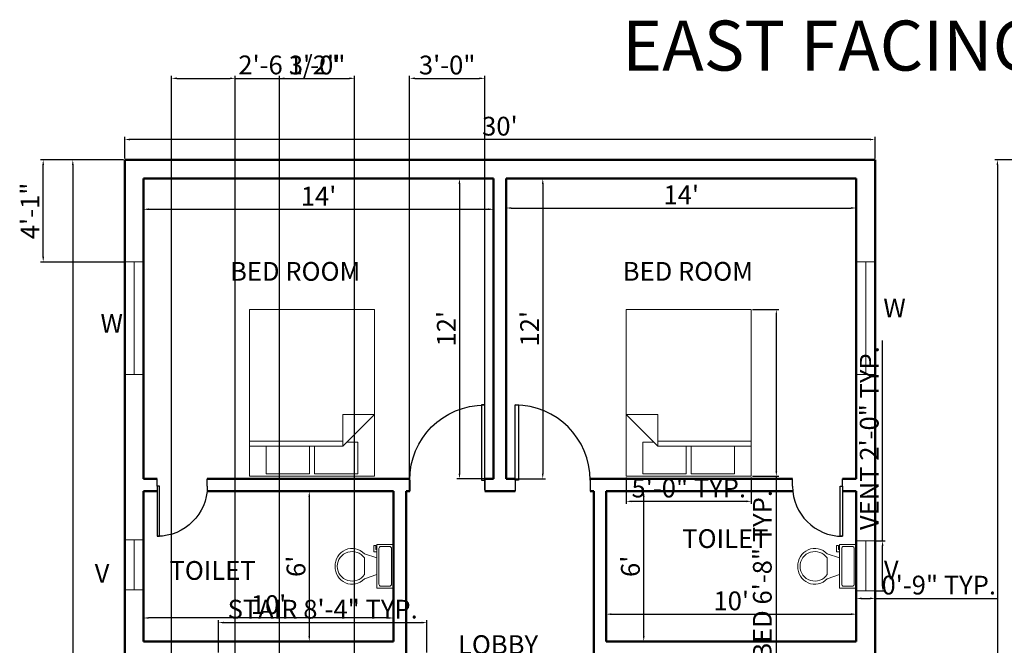
# Model space of a CAD drawing. Units: inches. Extents: x 3587 to 4539, y 1613 to 2440.
# Tile 6 of 8: x 3594 to 4067, y 2140 to 2440. Entities that reach past the tile are written whole.
import ezdxf

# ---------------------------------------------------------------- set-up
doc = ezdxf.new("R2010")
doc.units = ezdxf.units.IN
for name, color, linetype, lineweight in [('A-ANNO-DIMS', 2, 'Continuous', 18), ('A-ANNO-TEXT', 7, 'Continuous', 18), ('A-ANNO-TITL', 7, 'Continuous', 35), ('A-AREA-IDEN', 7, 'Continuous', 25), ('A-DOOR', 3, 'Continuous', 25), ('A-FLOR-FIXT', 9, 'Continuous', 18), ('A-FURN', 8, 'Continuous', 18), ('A-GLAZ', 4, 'Continuous', 20), ('A-WALL', 7, 'Continuous', 50)]:
    doc.layers.add(name, color=color, linetype=linetype, lineweight=lineweight)
doc.styles.get("Standard").update_dxf_attribs({"font": 'arial.ttf'})
doc.dimstyles.new('ISO-25', dxfattribs={"dimtxt": 9, "dimasz": 2.5, "dimexe": 1.25, "dimexo": 0.625, "dimtad": 1, "dimlunit": 3, "dimtxsty": 'Standard', "dimcen": 2.5, "dimadec": 0, "dimazin": 0, "dimtfac": 1, "dimtmove": 0, "dimatfit": 3, "dimfxl": 1, "dimarcsym": 0})

# ---------------------------------------------------------------- blocks, each defined once
blk = doc.blocks.new('*U4')
for p, q in [((0, 0), (0, -6)), ((40, 0), (40, -6))]:
    blk.add_line(p, q)
blk.add_lwpolyline([(0, 0), (0, 40), (1.75, 40), (1.75, 0)], close=True)
blk.add_arc((0, 0), 40, 0, 90)
blk = doc.blocks.new('*U11')
for p, q in [((9.5, -6), (9.5, -2)), ((-10, -8.5), (-8, -8.5)), ((-10, -9.5), (-10, -8.5)), ((-8, -8.5), (-8, -8)), ((-7, -8), (-7, -9.5)), ((-4, -8), (-6, -14)), ((4, -8), (6, -14)), ((-7, -9.5), (-10, -9.5)), ((4, -14), (-4, -14))]:
    blk.add_line(p, q)
blk.add_lwpolyline([(10.5, -8), (10.5, 0), (-10.5, 0), (-10.5, -8)], close=True)
for points in [[(-9.5, -2), (-9.5, -6)], [(8.5, -1), (-8.5, -1)], [(-8.5, -7), (8.5, -7)]]:
    blk.add_lwpolyline(points)
for centre, radius, start, end in [((-8.625, -1.875), 0.8839, 81.8699, 188.1301), ((8.625, -1.875), 0.8839, 351.8699, 98.1301), ((-8.625, -6.125), 0.8839, 171.869898, 278.1301), ((8.625, -6.125), 0.8839, 261.8699, 8.1301), ((-0.4772, -19.9188), 8.0953, 133.01722, 273.38), ((0.0374, -19.8731), 7.127, 124.50543, 269.7), ((-0.0373, -19.8731), 7.127, 270.3, 55.4946), ((0.4773, -19.9188), 8.0953, 266.62, 46.9828)]:
    blk.add_arc(centre, radius, start, end)
blk = doc.blocks.new('Bed - Queen')
for p, q in [((0, -80.00003), (0, 0)), ((0, 0), (59.99999, 0)), ((59.99999, 0), (59.99999, -80.00003)), ((7.99999, -1.2), (28.79998, -1.2)), ((7.99999, -14.4), (7.99999, -1.2)), ((28.79998, -1.2), (28.79998, -14.4)), ((31.19999, -1.2), (51.99999, -1.2)), ((31.19999, -14.4), (31.19999, -1.2)), ((51.99999, -1.2), (51.99999, -16.4)), ((0, -14.4), (44.8, -14.4)), ((44.8, -16.8), (0, -16.8)), ((59.99999, -29.6), (44.8, -14.4)), ((44.8, -14.4), (44.8, -29.6)), ((51.99999, -16.4), (46.79936, -16.4)), ((44.8, -29.6), (59.99999, -29.6)), ((59.99999, -80.00003), (0, -80.00003))]:
    blk.add_line(p, q)
blk = doc.blocks.new('*D13')
at = {"layer": 'A-ANNO-DIMS', "color": 0, "lineweight": -2, "transparency": 16777216}
for p, q in [((3644.52, 2373.56), (3644.52, 2383.96)), ((4002.02, 2382.71), (3647.02, 2382.71)), ((4004.52, 2373.56), (4004.52, 2383.96))]:
    blk.add_line(p, q, dxfattribs=at)
at = {"layer": 'A-ANNO-DIMS', "color": 0, "transparency": 16777216}
for points in [[(3647.02, 2383.12), (3647.02, 2382.29), (3644.52, 2382.71)], [(4002.02, 2383.12), (4002.02, 2382.29), (4004.52, 2382.71)]]:
    blk.add_solid(points, dxfattribs=at)
at = {"layer": 'Defpoints', "color": 0, "transparency": 16777216}
for p in [(3644.52, 2382.71), (3644.52, 2372.93), (4004.52, 2372.93)]:
    blk.add_point(p, dxfattribs=at)
at = {"layer": 'A-ANNO-DIMS', "color": 0, "transparency": 16777216, "insert": (3824.52, 2387.93), "char_height": 9, "attachment_point": 5}
blk.add_mtext("30'", dxfattribs=at)
blk = doc.blocks.new('*D14')
at = {"layer": 'A-ANNO-DIMS', "color": 0, "lineweight": -2, "transparency": 16777216}
for p, q in [((3643.9, 2372.93), (3618.39, 2372.93)), ((3619.64, 2370.43), (3619.64, 1655.43)), ((3643.9, 1652.93), (3618.39, 1652.93))]:
    blk.add_line(p, q, dxfattribs=at)
at = {"layer": 'A-ANNO-DIMS', "color": 0, "transparency": 16777216}
for points in [[(3619.22, 2370.43), (3620.05, 2370.43), (3619.64, 2372.93)], [(3619.22, 1655.43), (3620.05, 1655.43), (3619.64, 1652.93)]]:
    blk.add_solid(points, dxfattribs=at)
at = {"layer": 'Defpoints', "color": 0, "transparency": 16777216}
for p in [(3644.52, 2372.93), (3619.64, 1652.93), (3644.52, 1652.93)]:
    blk.add_point(p, dxfattribs=at)
at = {"layer": 'A-ANNO-DIMS', "color": 0, "transparency": 16777216, "insert": (3614.42, 2019.45), "char_height": 9, "attachment_point": 5, "rotation": 90}
blk.add_mtext("60'", dxfattribs=at)
blk = doc.blocks.new('*D15')
at = {"layer": 'A-ANNO-DIMS', "color": 0, "lineweight": -2, "transparency": 16777216}
for p, q in [((3653.52, 2363.31), (3653.52, 2347.98)), ((3821.52, 2363.31), (3821.52, 2347.98)), ((3656.02, 2349.23), (3819.02, 2349.23))]:
    blk.add_line(p, q, dxfattribs=at)
at = {"layer": 'A-ANNO-DIMS', "color": 0, "transparency": 16777216}
for points in [[(3656.02, 2349.64), (3656.02, 2348.81), (3653.52, 2349.23)], [(3819.02, 2349.64), (3819.02, 2348.81), (3821.52, 2349.23)]]:
    blk.add_solid(points, dxfattribs=at)
at = {"layer": 'Defpoints', "color": 0, "transparency": 16777216}
for p in [(3653.52, 2363.93), (3821.52, 2363.93), (3821.52, 2349.23)]:
    blk.add_point(p, dxfattribs=at)
at = {"layer": 'A-ANNO-DIMS', "color": 0, "transparency": 16777216, "insert": (3737.52, 2354.37), "char_height": 9, "attachment_point": 5}
blk.add_mtext("14'", dxfattribs=at)
blk = doc.blocks.new('*D16')
at = {"layer": 'A-ANNO-DIMS', "color": 0, "lineweight": -2, "transparency": 16777216}
for p, q in [((3820.9, 2363.93), (3803.88, 2363.93)), ((3805.13, 2361.43), (3805.13, 2222.43)), ((3820.9, 2219.93), (3803.88, 2219.93))]:
    blk.add_line(p, q, dxfattribs=at)
at = {"layer": 'A-ANNO-DIMS', "color": 0, "transparency": 16777216}
for points in [[(3804.72, 2361.43), (3805.55, 2361.43), (3805.13, 2363.93)], [(3804.72, 2222.43), (3805.55, 2222.43), (3805.13, 2219.93)]]:
    blk.add_solid(points, dxfattribs=at)
at = {"layer": 'Defpoints', "color": 0, "transparency": 16777216}
for p in [(3821.52, 2363.93), (3805.13, 2219.93), (3821.52, 2219.93)]:
    blk.add_point(p, dxfattribs=at)
at = {"layer": 'A-ANNO-DIMS', "color": 0, "transparency": 16777216, "insert": (3799.99, 2291.93), "char_height": 9, "attachment_point": 5, "rotation": 90}
blk.add_mtext("12'", dxfattribs=at)
blk = doc.blocks.new('*D17')
at = {"layer": 'A-ANNO-DIMS', "color": 0, "lineweight": -2, "transparency": 16777216}
for p, q in [((3827.52, 2363.31), (3827.52, 2348.58)), ((3995.52, 2363.31), (3995.52, 2348.58)), ((3830.02, 2349.83), (3993.02, 2349.83))]:
    blk.add_line(p, q, dxfattribs=at)
at = {"layer": 'A-ANNO-DIMS', "color": 0, "transparency": 16777216}
for points in [[(3830.02, 2350.25), (3830.02, 2349.41), (3827.52, 2349.83)], [(3993.02, 2350.25), (3993.02, 2349.41), (3995.52, 2349.83)]]:
    blk.add_solid(points, dxfattribs=at)
at = {"layer": 'Defpoints', "color": 0, "transparency": 16777216}
for p in [(3827.52, 2363.93), (3995.52, 2363.93), (3995.52, 2349.83)]:
    blk.add_point(p, dxfattribs=at)
at = {"layer": 'A-ANNO-DIMS', "color": 0, "transparency": 16777216, "insert": (3911.52, 2354.97), "char_height": 9, "attachment_point": 5}
blk.add_mtext("14'", dxfattribs=at)
blk = doc.blocks.new('*D18')
at = {"layer": 'A-ANNO-DIMS', "color": 0, "lineweight": -2, "transparency": 16777216}
for p, q in [((3828.15, 2363.93), (3846.35, 2363.93)), ((3845.1, 2361.43), (3845.1, 2222.43)), ((3828.15, 2219.93), (3846.35, 2219.93))]:
    blk.add_line(p, q, dxfattribs=at)
at = {"layer": 'A-ANNO-DIMS', "color": 0, "transparency": 16777216}
for points in [[(3844.68, 2361.43), (3845.51, 2361.43), (3845.1, 2363.93)], [(3844.68, 2222.43), (3845.51, 2222.43), (3845.1, 2219.93)]]:
    blk.add_solid(points, dxfattribs=at)
at = {"layer": 'Defpoints', "color": 0, "transparency": 16777216}
for p in [(3827.52, 2363.93), (3827.52, 2219.93), (3845.1, 2219.93)]:
    blk.add_point(p, dxfattribs=at)
at = {"layer": 'A-ANNO-DIMS', "color": 0, "transparency": 16777216, "insert": (3839.95, 2291.93), "char_height": 9, "attachment_point": 5, "rotation": 90}
blk.add_mtext("12'", dxfattribs=at)
blk = doc.blocks.new('*D19')
at = {"layer": 'A-ANNO-DIMS', "color": 0, "lineweight": -2, "transparency": 16777216}
for p, q in [((3653.52, 2142.56), (3653.52, 2154.41)), ((3773.52, 2142.56), (3773.52, 2154.41)), ((3771.02, 2153.16), (3656.02, 2153.16))]:
    blk.add_line(p, q, dxfattribs=at)
at = {"layer": 'A-ANNO-DIMS', "color": 0, "transparency": 16777216}
for points in [[(3656.02, 2153.58), (3656.02, 2152.75), (3653.52, 2153.16)], [(3771.02, 2153.58), (3771.02, 2152.75), (3773.52, 2153.16)]]:
    blk.add_solid(points, dxfattribs=at)
at = {"layer": 'Defpoints', "color": 0, "transparency": 16777216}
for p in [(3653.52, 2153.16), (3653.52, 2141.93), (3773.52, 2141.93)]:
    blk.add_point(p, dxfattribs=at)
at = {"layer": 'A-ANNO-DIMS', "color": 0, "transparency": 16777216, "insert": (3713.52, 2158.38), "char_height": 9, "attachment_point": 5}
blk.add_mtext("10'", dxfattribs=at)
blk = doc.blocks.new('*D20')
at = {"layer": 'A-ANNO-DIMS', "color": 0, "lineweight": -2, "transparency": 16777216}
for p, q in [((3772.9, 2213.93), (3731.83, 2213.93)), ((3733.08, 2211.43), (3733.08, 2144.43)), ((3772.9, 2141.93), (3731.83, 2141.93))]:
    blk.add_line(p, q, dxfattribs=at)
at = {"layer": 'A-ANNO-DIMS', "color": 0, "transparency": 16777216}
for points in [[(3732.67, 2211.43), (3733.5, 2211.43), (3733.08, 2213.93)], [(3732.67, 2144.43), (3733.5, 2144.43), (3733.08, 2141.93)]]:
    blk.add_solid(points, dxfattribs=at)
at = {"layer": 'Defpoints', "color": 0, "transparency": 16777216}
for p in [(3773.52, 2213.93), (3733.08, 2141.93), (3773.52, 2141.93)]:
    blk.add_point(p, dxfattribs=at)
at = {"layer": 'A-ANNO-DIMS', "color": 0, "transparency": 16777216, "insert": (3727.86, 2177.93), "char_height": 9, "attachment_point": 5, "rotation": 90}
blk.add_mtext("6'", dxfattribs=at)
blk = doc.blocks.new('*D21')
at = {"layer": 'A-ANNO-DIMS', "color": 0, "lineweight": -2, "transparency": 16777216}
for p, q in [((3876.15, 2213.93), (3894.78, 2213.93)), ((3893.53, 2144.43), (3893.53, 2211.43)), ((3876.15, 2141.93), (3894.78, 2141.93))]:
    blk.add_line(p, q, dxfattribs=at)
at = {"layer": 'A-ANNO-DIMS', "color": 0, "transparency": 16777216}
for points in [[(3893.12, 2211.43), (3893.95, 2211.43), (3893.53, 2213.93)], [(3893.12, 2144.43), (3893.95, 2144.43), (3893.53, 2141.93)]]:
    blk.add_solid(points, dxfattribs=at)
at = {"layer": 'Defpoints', "color": 0, "transparency": 16777216}
for p in [(3875.52, 2213.93), (3893.53, 2213.93), (3875.52, 2141.93)]:
    blk.add_point(p, dxfattribs=at)
at = {"layer": 'A-ANNO-DIMS', "color": 0, "transparency": 16777216, "insert": (3888.31, 2177.93), "char_height": 9, "attachment_point": 5, "rotation": 90}
blk.add_mtext("6'", dxfattribs=at)
blk = doc.blocks.new('*D22')
at = {"layer": 'A-ANNO-DIMS', "color": 0, "lineweight": -2, "transparency": 16777216}
for p, q in [((3875.52, 2142.56), (3875.52, 2156.23)), ((3878.02, 2154.98), (3993.02, 2154.98)), ((3995.52, 2142.56), (3995.52, 2156.23))]:
    blk.add_line(p, q, dxfattribs=at)
at = {"layer": 'A-ANNO-DIMS', "color": 0, "transparency": 16777216}
for points in [[(3878.02, 2155.4), (3878.02, 2154.56), (3875.52, 2154.98)], [(3993.02, 2155.4), (3993.02, 2154.56), (3995.52, 2154.98)]]:
    blk.add_solid(points, dxfattribs=at)
at = {"layer": 'Defpoints', "color": 0, "transparency": 16777216}
for p in [(3995.52, 2154.98), (3875.52, 2141.93), (3995.52, 2141.93)]:
    blk.add_point(p, dxfattribs=at)
at = {"layer": 'A-ANNO-DIMS', "color": 0, "transparency": 16777216, "insert": (3935.52, 2160.2), "char_height": 9, "attachment_point": 5}
blk.add_mtext("10'", dxfattribs=at)
blk = doc.blocks.new('*D28')
at = {"layer": 'A-ANNO-DIMS', "color": 0, "lineweight": -2, "transparency": 16777216}
for p, q in [((4087.49, 2372.93), (4061.98, 2372.93)), ((4063.23, 2370.43), (4063.23, 1655.43)), ((4087.49, 1652.93), (4061.98, 1652.93))]:
    blk.add_line(p, q, dxfattribs=at)
at = {"layer": 'A-ANNO-DIMS', "color": 0, "transparency": 16777216}
for points in [[(4062.81, 2370.43), (4063.65, 2370.43), (4063.23, 2372.93)], [(4062.81, 1655.43), (4063.65, 1655.43), (4063.23, 1652.93)]]:
    blk.add_solid(points, dxfattribs=at)
at = {"layer": 'Defpoints', "color": 0, "transparency": 16777216}
for p in [(4088.12, 2372.93), (4063.23, 1652.93), (4088.12, 1652.93)]:
    blk.add_point(p, dxfattribs=at)
at = {"layer": 'A-ANNO-DIMS', "color": 0, "transparency": 16777216, "insert": (4058.01, 2019.45), "char_height": 9, "attachment_point": 5, "rotation": 90}
blk.add_mtext("60'", dxfattribs=at)
blk = doc.blocks.new('WINDOW-54IN')
for p, q in [((9, 54), (0, 54)), ((4.5, 54), (4.5, 0)), ((9, 0), (0, 0))]:
    blk.add_line(p, q)
blk = doc.blocks.new('VENT-24IN')
for p, q in [((9, 24), (0, 24)), ((4.5, 0), (4.5, 24)), ((9, 0), (0, 0))]:
    blk.add_line(p, q)
blk = doc.blocks.new('*D56')
at = {"layer": 'A-ANNO-DIMS', "color": 0, "lineweight": -2, "transparency": 16777216}
for p, q in [((4008.12, 2190.14), (4008.12, 2286.24)), ((4005.15, 2190.14), (4009.37, 2190.14)), ((4008.12, 2168.64), (4008.12, 2187.64)), ((4005.15, 2166.14), (4009.37, 2166.14))]:
    blk.add_line(p, q, dxfattribs=at)
at = {"layer": 'A-ANNO-DIMS', "color": 0, "transparency": 16777216}
for points in [[(4007.71, 2187.64), (4008.54, 2187.64), (4008.12, 2190.14)], [(4007.71, 2168.64), (4008.54, 2168.64), (4008.12, 2166.14)]]:
    blk.add_solid(points, dxfattribs=at)
at = {"layer": 'Defpoints', "color": 0, "transparency": 16777216}
for p in [(4004.52, 2190.14), (4008.12, 2190.14), (4004.52, 2166.14)]:
    blk.add_point(p, dxfattribs=at)
at = {"layer": 'A-ANNO-DIMS', "color": 0, "transparency": 16777216, "insert": (4002.9, 2239.44), "char_height": 9, "attachment_point": 5, "rotation": 90}
blk.add_mtext('VENT 2\'-0" TYP.', dxfattribs=at)
blk = doc.blocks.new('*D57')
at = {"layer": 'A-ANNO-DIMS', "color": 0, "lineweight": -2, "transparency": 16777216}
for p, q in [((3995.52, 2165.51), (3995.52, 2161.29)), ((4004.52, 2165.51), (4004.52, 2161.29)), ((3998.02, 2162.54), (4002.02, 2162.54)), ((4004.52, 2162.54), (4063.13, 2162.54))]:
    blk.add_line(p, q, dxfattribs=at)
at = {"layer": 'A-ANNO-DIMS', "color": 0, "transparency": 16777216}
for points in [[(3998.02, 2162.95), (3998.02, 2162.12), (3995.52, 2162.54)], [(4002.02, 2162.95), (4002.02, 2162.12), (4004.52, 2162.54)]]:
    blk.add_solid(points, dxfattribs=at)
at = {"layer": 'Defpoints', "color": 0, "transparency": 16777216}
for p in [(3995.52, 2166.14), (4004.52, 2166.14), (4004.52, 2162.54)]:
    blk.add_point(p, dxfattribs=at)
at = {"layer": 'A-ANNO-DIMS', "color": 0, "transparency": 16777216, "insert": (4035.08, 2167.76), "char_height": 9, "attachment_point": 5}
blk.add_mtext('0\'-9" TYP.', dxfattribs=at)
blk = doc.blocks.new('*D60')
at = {"layer": 'A-ANNO-DIMS', "color": 0, "lineweight": -2, "transparency": 16777216}
for p, q in [((3945.78, 2301.11), (3958.4, 2301.11)), ((3957.15, 2298.61), (3957.15, 2223.61)), ((3945.78, 2221.11), (3958.4, 2221.11)), ((3957.15, 2221.11), (3957.15, 2084.97))]:
    blk.add_line(p, q, dxfattribs=at)
at = {"layer": 'A-ANNO-DIMS', "color": 0, "transparency": 16777216}
for points in [[(3956.74, 2298.61), (3957.57, 2298.61), (3957.15, 2301.11)], [(3956.74, 2223.61), (3957.57, 2223.61), (3957.15, 2221.11)]]:
    blk.add_solid(points, dxfattribs=at)
at = {"layer": 'Defpoints', "color": 0, "transparency": 16777216}
for p in [(3945.15, 2301.11), (3945.15, 2221.11), (3957.15, 2221.11)]:
    blk.add_point(p, dxfattribs=at)
at = {"layer": 'A-ANNO-DIMS', "color": 0, "transparency": 16777216, "insert": (3951.6, 2151.79), "char_height": 9, "attachment_point": 5, "rotation": 90}
blk.add_mtext('QUEEN BED 6\'-8" TYP.', dxfattribs=at)
blk = doc.blocks.new('*D61')
at = {"layer": 'A-ANNO-DIMS', "color": 0, "lineweight": -2, "transparency": 16777216}
for p, q in [((3885.15, 2220.49), (3885.15, 2207.86)), ((3945.15, 2220.49), (3945.15, 2207.86)), ((3942.65, 2209.11), (3887.65, 2209.11))]:
    blk.add_line(p, q, dxfattribs=at)
at = {"layer": 'A-ANNO-DIMS', "color": 0, "transparency": 16777216}
for points in [[(3887.65, 2209.53), (3887.65, 2208.69), (3885.15, 2209.11)], [(3942.65, 2209.53), (3942.65, 2208.69), (3945.15, 2209.11)]]:
    blk.add_solid(points, dxfattribs=at)
at = {"layer": 'Defpoints', "color": 0, "transparency": 16777216}
for p in [(3885.15, 2221.11), (3945.15, 2221.11), (3885.15, 2209.11)]:
    blk.add_point(p, dxfattribs=at)
at = {"layer": 'A-ANNO-DIMS', "color": 0, "transparency": 16777216, "insert": (3915.15, 2214.33), "char_height": 9, "attachment_point": 5}
blk.add_mtext('5\'-0" TYP.', dxfattribs=at)
blk = doc.blocks.new('*D66')
at = {"layer": 'A-ANNO-DIMS', "color": 0, "lineweight": -2, "transparency": 16777216}
for p, q in [((3689.52, 2136.56), (3689.52, 2152.18)), ((3692.02, 2150.93), (3787.02, 2150.93)), ((3789.52, 2136.56), (3789.52, 2152.18))]:
    blk.add_line(p, q, dxfattribs=at)
at = {"layer": 'A-ANNO-DIMS', "color": 0, "transparency": 16777216}
for points in [[(3692.02, 2151.35), (3692.02, 2150.52), (3689.52, 2150.93)], [(3787.02, 2151.35), (3787.02, 2150.52), (3789.52, 2150.93)]]:
    blk.add_solid(points, dxfattribs=at)
at = {"layer": 'Defpoints', "color": 0, "transparency": 16777216}
for p in [(3789.52, 2150.93), (3689.52, 2135.93), (3789.52, 2135.93)]:
    blk.add_point(p, dxfattribs=at)
at = {"layer": 'A-ANNO-DIMS', "color": 0, "transparency": 16777216, "insert": (3739.52, 2156.21), "char_height": 9, "attachment_point": 5}
blk.add_mtext('STAIR 8\'-4" TYP.', dxfattribs=at)
blk = doc.blocks.new('*D91')
at = {"layer": 'A-ANNO-DIMS', "color": 0, "lineweight": -2, "transparency": 16777216}
for p, q in [((3781.24, 2214.56), (3781.24, 2413.28)), ((3783.74, 2412.03), (3814.74, 2412.03)), ((3817.24, 2214.56), (3817.24, 2413.28))]:
    blk.add_line(p, q, dxfattribs=at)
at = {"layer": 'A-ANNO-DIMS', "color": 0, "transparency": 16777216}
for points in [[(3783.74, 2412.45), (3783.74, 2411.62), (3781.24, 2412.03)], [(3814.74, 2412.45), (3814.74, 2411.62), (3817.24, 2412.03)]]:
    blk.add_solid(points, dxfattribs=at)
at = {"layer": 'Defpoints', "color": 0, "transparency": 16777216}
for p in [(3817.24, 2412.03), (3781.24, 2213.93), (3817.24, 2213.93)]:
    blk.add_point(p, dxfattribs=at)
at = {"layer": 'A-ANNO-DIMS', "color": 0, "transparency": 16777216, "insert": (3799.24, 2417.26), "char_height": 9, "attachment_point": 5}
blk.add_mtext('3\'-0"', dxfattribs=at)
blk = doc.blocks.new('*D92')
at = {"layer": 'A-ANNO-DIMS', "color": 0, "lineweight": -2, "transparency": 16777216}
for p, q in [((3643.9, 2372.93), (3604.17, 2372.93)), ((3605.42, 2326.43), (3605.42, 2370.43)), ((3643.9, 2323.93), (3604.17, 2323.93))]:
    blk.add_line(p, q, dxfattribs=at)
at = {"layer": 'A-ANNO-DIMS', "color": 0, "transparency": 16777216}
for points in [[(3605.01, 2370.43), (3605.84, 2370.43), (3605.42, 2372.93)], [(3605.01, 2326.43), (3605.84, 2326.43), (3605.42, 2323.93)]]:
    blk.add_solid(points, dxfattribs=at)
at = {"layer": 'Defpoints', "color": 0, "transparency": 16777216}
for p in [(3605.42, 2372.93), (3644.52, 2372.93), (3644.52, 2323.93)]:
    blk.add_point(p, dxfattribs=at)
at = {"layer": 'A-ANNO-DIMS', "color": 0, "transparency": 16777216, "insert": (3600.28, 2348.43), "char_height": 9, "attachment_point": 5, "rotation": 90}
blk.add_mtext('4\'-1"', dxfattribs=at)
blk = doc.blocks.new('*D96')
at = {"layer": 'A-ANNO-DIMS', "color": 0, "lineweight": -2, "transparency": 16777216}
for p, q in [((3667.04, 1858.35), (3667.04, 2413.28)), ((3669.54, 2412.03), (3695.05, 2412.03)), ((3697.55, 1858.35), (3697.55, 2413.28)), ((3697.55, 2412.03), (3746.35, 2412.03))]:
    blk.add_line(p, q, dxfattribs=at)
at = {"layer": 'A-ANNO-DIMS', "color": 0, "transparency": 16777216}
for points in [[(3669.54, 2412.45), (3669.54, 2411.62), (3667.04, 2412.03)], [(3695.05, 2412.45), (3695.05, 2411.62), (3697.55, 2412.03)]]:
    blk.add_solid(points, dxfattribs=at)
at = {"layer": 'Defpoints', "color": 0, "transparency": 16777216}
for p in [(3697.55, 2412.03), (3667.04, 1857.73), (3697.55, 1857.73)]:
    blk.add_point(p, dxfattribs=at)
at = {"layer": 'A-ANNO-DIMS', "color": 0, "transparency": 16777216, "insert": (3723.2, 2417.31), "char_height": 9, "attachment_point": 5}
blk.add_mtext('2\'-6 1/2"', dxfattribs=at)
blk = doc.blocks.new('*D98')
at = {"layer": 'A-ANNO-DIMS', "color": 0, "lineweight": -2, "transparency": 16777216}
for p, q in [((3718.85, 1857.52), (3718.85, 2413.28)), ((3721.35, 2412.03), (3752.35, 2412.03)), ((3754.85, 1857.52), (3754.85, 2413.28))]:
    blk.add_line(p, q, dxfattribs=at)
at = {"layer": 'A-ANNO-DIMS', "color": 0, "transparency": 16777216}
for points in [[(3721.35, 2412.45), (3721.35, 2411.62), (3718.85, 2412.03)], [(3752.35, 2412.45), (3752.35, 2411.62), (3754.85, 2412.03)]]:
    blk.add_solid(points, dxfattribs=at)
at = {"layer": 'Defpoints', "color": 0, "transparency": 16777216}
for p in [(3754.85, 2412.03), (3718.85, 1856.9), (3754.85, 1856.9)]:
    blk.add_point(p, dxfattribs=at)
at = {"layer": 'A-ANNO-DIMS', "color": 0, "transparency": 16777216, "insert": (3736.85, 2417.26), "char_height": 9, "attachment_point": 5}
blk.add_mtext('3\'-0"', dxfattribs=at)

msp = doc.modelspace()

# ---------------------------------------------------------------- linework, layer by layer
at = {"layer": 'A-WALL'}
for p, q in [((4004.523, 2372.933), (3644.523, 2372.933)), ((3644.523, 2372.933), (3644.523, 1652.933)), ((4004.523, 2372.933), (4004.523, 1652.933)), ((3653.523, 2363.933), (3653.523, 2219.933)), ((3821.523, 2363.933), (3653.523, 2363.933)), ((3821.523, 2363.933), (3821.523, 2219.933)), ((3995.523, 2363.933), (3827.523, 2363.933)), ((3827.523, 2363.933), (3827.523, 2219.933)), ((3995.523, 2363.933), (3995.523, 2219.933)), ((3660.14, 2219.933), (3653.523, 2219.933)), ((3781.248, 2219.933), (3684.14, 2219.933)), ((3821.523, 2219.933), (3817.243, 2219.933)), ((3831.804, 2219.933), (3827.523, 2219.933)), ((3964.907, 2219.933), (3867.799, 2219.933)), ((3995.523, 2219.933), (3988.907, 2219.933)), ((3653.523, 2213.933), (3653.523, 2141.933)), ((3660.14, 2213.933), (3653.523, 2213.933)), ((3773.523, 2213.933), (3684.02, 2213.933)), ((3773.523, 2213.933), (3773.523, 2141.933)), ((3779.523, 2213.933), (3779.523, 2135.933)), ((3781.243, 2213.933), (3779.523, 2213.933)), ((3821.523, 2213.933), (3817.243, 2213.933)), ((3831.804, 2213.933), (3821.523, 2213.933)), ((3869.523, 2213.933), (3867.804, 2213.933)), ((3869.523, 2213.933), (3869.523, 2135.933)), ((3875.523, 2213.933), (3875.523, 2141.933)), ((3965.027, 2213.933), (3875.523, 2213.933)), ((3995.523, 2213.933), (3988.907, 2213.933)), ((3995.523, 2213.933), (3995.523, 2141.933)), ((3773.523, 2141.933), (3653.523, 2141.933)), ((3995.523, 2141.933), (3875.523, 2141.933))]:
    msp.add_line(p, q, dxfattribs=at)

# ---------------------------------------------------------------- block references
at = {"layer": 'A-DOOR', "yscale": 0.9, "zscale": 0.9}
for p, xscale in [((3817.243, 2219.333), -0.9), ((3831.804, 2219.333), 0.9)]:
    msp.add_blockref('*U4', p, dxfattribs=dict(at, xscale=xscale))
at = {"layer": 'A-DOOR', "yscale": 0.6, "zscale": 0.6, "rotation": 180}
for p, xscale in [((3660.14, 2216.333), -0.6), ((3988.907, 2216.333), 0.6)]:
    msp.add_blockref('*U4', p, dxfattribs=dict(at, xscale=xscale))
at = {"layer": 'A-FLOR-FIXT', "rotation": 270}
for p in [(3773.523, 2177.933), (3995.523, 2177.933)]:
    msp.add_blockref('*U11', p, dxfattribs=at)
at = {"layer": 'A-FURN', "xscale": -1, "rotation": 180}
msp.add_blockref('Bed - Queen', (3704.324, 2221.11), dxfattribs=at)
at = {"layer": 'A-FURN', "rotation": 180}
msp.add_blockref('Bed - Queen', (3945.153, 2221.11), dxfattribs=at)
at = {"layer": 'A-GLAZ'}
for name, p in [('WINDOW-54IN', (3644.523, 2269.932)), ('WINDOW-54IN', (3995.523, 2269.932)), ('VENT-24IN', (3644.523, 2166.578)), ('VENT-24IN', (3995.523, 2166.139))]:
    msp.add_blockref(name, p, dxfattribs=at)

# ---------------------------------------------------------------- texts
at = {"layer": 'A-ANNO-TEXT', "char_height": 9, "attachment_point": 1}
for s, width, insert in [('W', 47.85632, (4008.481, 2306.421)), ('W', 47.85632, (3632.896, 2299.001)), ('V', 55.41427, (3630.132, 2179.076)), ('V', 55.41427, (4008.752, 2180.666))]:
    msp.add_mtext_dynamic_manual_height_columns(s, width=width, gutter_width=12.5, heights=[0], dxfattribs=dict(at, insert=insert))
at = {"layer": 'A-ANNO-TITL', "insert": (3883.118, 2439.751), "char_height": 24, "attachment_point": 1}
msp.add_mtext_dynamic_manual_height_columns('EAST FACING HOUSE', width=425.00601, gutter_width=12.5, heights=[0], dxfattribs=at)
at = {"layer": 'A-AREA-IDEN', "char_height": 9, "attachment_point": 1}
for s, width, insert in [('BED ROOM', 136.86909, (3695.081, 2323.938)), ('BED ROOM', 136.86909, (3883.472, 2323.95)), ('TOILET', 135.91196, (3912.02, 2195.74)), ('TOILET', 135.91196, (3666.028, 2180.453)), ('LOBBY', 107.19817, (3804.425, 2144.864))]:
    msp.add_mtext_dynamic_manual_height_columns(s, width=width, gutter_width=12.5, heights=[0], dxfattribs=dict(at, insert=insert))

# ---------------------------------------------------------------- dimensions: what is measured, and where the dimension line sits
at = {"layer": 'A-ANNO-DIMS'}
for base, p1, p2, override, picture, middle in [((3697.551, 2412.033), (3667.042, 1857.729), (3697.551, 1857.729), {"dimdec": 1, "dimlfac": 1, "dimrnd": 0, "dimzin": 1, "dimdsep": 46, "dimlunit": 4, "dimfrac": 2}, '*D96', (3723.2, 2417.312)), ((3754.854, 2412.033), (3718.854, 1856.898), (3754.854, 1856.898), {"dimdec": 1, "dimlfac": 1, "dimrnd": 0, "dimzin": 1, "dimdsep": 46, "dimlunit": 4, "dimfrac": 2}, '*D98', (3736.854, 2417.256)), ((3817.243, 2412.033), (3781.243, 2213.933), (3817.243, 2213.933), {"dimdec": 1, "dimlfac": 1, "dimrnd": 0, "dimzin": 1, "dimdsep": 46, "dimlunit": 4, "dimfrac": 2}, '*D91', (3799.243, 2417.256)), ((3644.523, 2382.707), (4004.523, 2372.933), (3644.523, 2372.933), {"dimclrd": 0, "dimclre": 0, "dimclrt": 0}, '*D13', (3824.523, 2387.93)), ((3821.523, 2349.226), (3653.523, 2363.933), (3821.523, 2363.933), {"dimclrd": 0, "dimclre": 0, "dimclrt": 0}, '*D15', (3737.523, 2354.37)), ((3995.523, 2349.831), (3827.523, 2363.933), (3995.523, 2363.933), {"dimclrd": 0, "dimclre": 0, "dimclrt": 0}, '*D17', (3911.523, 2354.975)), ((3653.523, 2153.164), (3773.523, 2141.933), (3653.523, 2141.933), {"dimclrd": 0, "dimclre": 0, "dimclrt": 0}, '*D19', (3713.523, 2158.384)), ((3995.523, 2154.979), (3875.523, 2141.933), (3995.523, 2141.933), {"dimclrd": 0, "dimclre": 0, "dimclrt": 0}, '*D22', (3935.523, 2160.2))]:
    dim = msp.add_linear_dim(base=base, p1=p1, p2=p2, dimstyle='ISO-25', override=override, dxfattribs=at)
    dim.commit()
    dim.dimension.update_dxf_attribs({"geometry": picture, "text_midpoint": middle})
for base, p1, p2, override, picture, middle in [((3605.423, 2372.933), (3644.523, 2323.932), (3644.523, 2372.933), {"dimdec": 1, "dimlfac": 1, "dimrnd": 0, "dimzin": 1, "dimdsep": 46, "dimlunit": 4, "dimfrac": 2}, '*D92', (3600.28, 2348.432)), ((3805.135, 2219.933), (3821.523, 2363.933), (3821.523, 2219.933), {"dimclrd": 0, "dimclre": 0, "dimclrt": 0}, '*D16', (3799.992, 2291.933)), ((3845.096, 2219.933), (3827.523, 2363.933), (3827.523, 2219.933), {"dimclrd": 0, "dimclre": 0, "dimclrt": 0}, '*D18', (3839.952, 2291.933)), ((3733.085, 2141.933), (3773.523, 2213.933), (3773.523, 2141.933), {"dimclrd": 0, "dimclre": 0, "dimclrt": 0}, '*D20', (3727.864, 2177.933)), ((3893.533, 2213.933), (3875.523, 2141.933), (3875.523, 2213.933), {"dimclrd": 0, "dimclre": 0, "dimclrt": 0}, '*D21', (3888.313, 2177.933))]:
    dim = msp.add_linear_dim(base=base, p1=p1, p2=p2, angle=90, dimstyle='ISO-25', override=override, dxfattribs=at)
    dim.commit()
    dim.dimension.update_dxf_attribs({"geometry": picture, "text_midpoint": middle})
for base, p1, p2, picture, middle in [((3619.637, 1652.933), (3644.523, 2372.933), (3644.523, 1652.933), '*D14', (3619.637, 2019.453)), ((4063.23, 1652.933), (4088.116, 2372.933), (4088.116, 1652.933), '*D28', (4063.23, 2019.453))]:
    dim = msp.add_linear_dim(base=base, p1=p1, p2=p2, angle=90, dimstyle='ISO-25', override={"dimclrd": 0, "dimclre": 0, "dimclrt": 0}, dxfattribs=at)
    dim.commit()
    dim.dimension.update_dxf_attribs({"geometry": picture, "text_midpoint": middle, "dimtype": 160})
for base, p1, p2, angle, text, picture, middle in [((3957.153, 2221.11), (3945.153, 2301.11), (3945.153, 2221.11), 270, 'QUEEN BED <> TYP.', '*D60', (3951.598, 2151.79)), ((4008.123, 2190.138), (4004.523, 2166.138), (4004.523, 2190.138), 90, 'VENT <> TYP.', '*D56', (4002.903, 2239.439)), ((3885.153, 2209.11), (3945.153, 2221.11), (3885.153, 2221.11), 180, '<> TYP.', '*D61', (3915.153, 2214.331))]:
    dim = msp.add_linear_dim(base=base, p1=p1, p2=p2, angle=angle, text=text, dimstyle='ISO-25', override={"dimdec": 1, "dimlfac": 1, "dimrnd": 0, "dimzin": 1, "dimdsep": 46, "dimlunit": 4, "dimfrac": 2}, dxfattribs=at)
    dim.commit()
    dim.dimension.update_dxf_attribs({"geometry": picture, "text_midpoint": middle})
for base, p1, p2, text, picture, middle in [((4004.523, 2162.538), (3995.523, 2166.138), (4004.523, 2166.138), '<> TYP.', '*D57', (4035.078, 2167.758)), ((3789.523, 2150.933), (3689.523, 2135.933), (3789.523, 2135.933), 'STAIR <> TYP.', '*D66', (3739.523, 2156.212))]:
    dim = msp.add_linear_dim(base=base, p1=p1, p2=p2, text=text, dimstyle='ISO-25', override={"dimdec": 1, "dimlfac": 1, "dimrnd": 0, "dimzin": 1, "dimdsep": 46, "dimlunit": 4, "dimfrac": 2}, dxfattribs=at)
    dim.commit()
    dim.dimension.update_dxf_attribs({"geometry": picture, "text_midpoint": middle})

doc.saveas('drawing.dxf')
